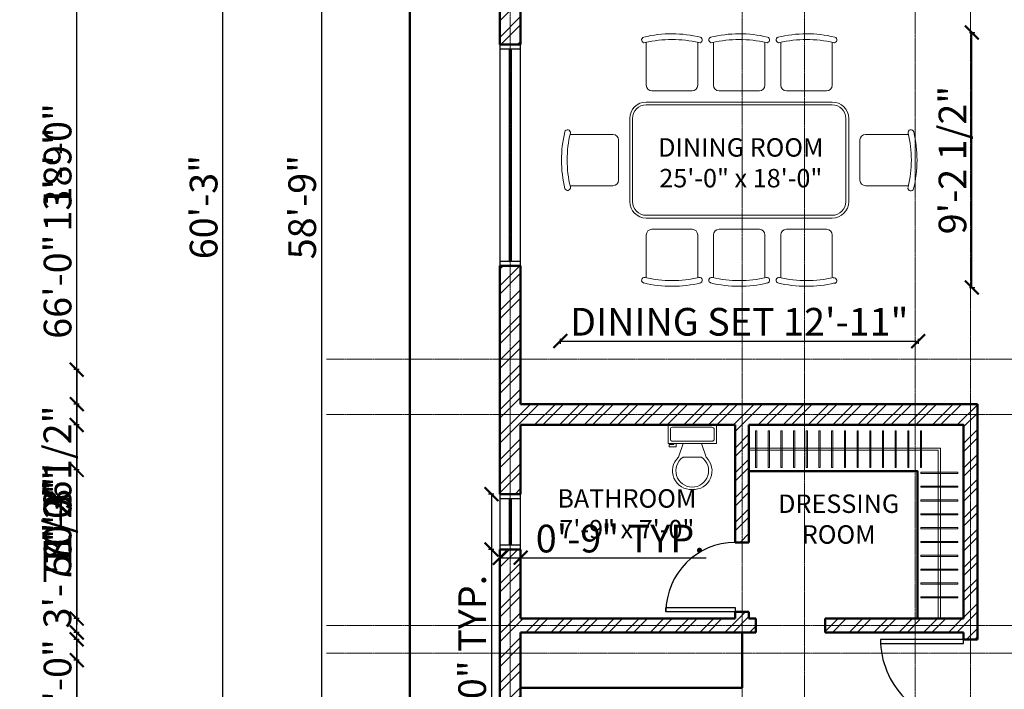
# Model space of a CAD drawing. Units: inches. Extents: x 261 to 2725, y 291 to 1454.
# Tile 6 of 35: x 261 to 688, y 661 to 951. Entities that reach past the tile are written whole.
import ezdxf

# ---------------------------------------------------------------- set-up
doc = ezdxf.new("R2010")
doc.units = ezdxf.units.IN
doc.linetypes.add('CENTER', pattern=[2, 1.25, -0.25, 0.25, -0.25])
for name, color, linetype, lineweight in [('A-ANNO-DIMS', 136, 'Continuous', 18), ('A-AREA-IDEN', 18, 'Continuous', 18), ('A-DOOR', 160, 'Continuous', 25), ('A-FLOR-FIXT', 145, 'Continuous', 18), ('A-FURN', 30, 'Continuous', 18), ('A-GLAZ', 150, 'Continuous', 25), ('A-GRID', 251, 'CENTER', 13), ('A-WALL', 222, 'Continuous', 50), ('A-WALL-PATT', 243, 'Continuous', 13)]:
    doc.layers.add(name, color=color, linetype=linetype, lineweight=lineweight)
doc.styles.get("Standard").update_dxf_attribs({"font": 'arial.ttf'})
doc.dimstyles.new('ISO-25', dxfattribs={"dimtxt": 12, "dimasz": 6, "dimexe": 1.25, "dimexo": 0.625, "dimtad": 1, "dimdec": 0, "dimlunit": 3, "dimtxsty": 'Standard', "dimblk": 'ARCHTICK', "dimcen": 2.5, "dimadec": 0, "dimazin": 0, "dimtfac": 1, "dimtdec": 0, "dimtmove": 0, "dimatfit": 3, "dimfxl": 1, "dimfxlon": 1, "dimarcsym": 0})

# ---------------------------------------------------------------- blocks, each defined once
blk = doc.blocks.new('*U5')
for p, q in [((0, 0), (0, -4)), ((-36, 0), (-36, -4))]:
    blk.add_line(p, q)
blk.add_lwpolyline([(0, 0), (0, 36), (-1.75, 36), (-1.75, 0)], close=True)
blk.add_arc((0, 0), 36, 90, 180)
blk = doc.blocks.new('*U3')
for p, q in [((0, 0), (0, -6)), ((30, 0), (30, -6))]:
    blk.add_line(p, q)
blk.add_lwpolyline([(0, 0), (0, 30), (1.75, 30), (1.75, 0)], close=True)
blk.add_arc((0, 0), 30, 0, 90)
blk = doc.blocks.new('A$C593F2FDE')
for p, q in [((0.8501, 2.0223), (0.8501, 2.4542)), ((1.3676, 2.0223), (1.3676, 2.4542)), ((1.5273, 2.0223), (1.5273, 2.4542)), ((2.0448, 2.0223), (2.0448, 2.4542)), ((2.2045, 2.0223), (2.2045, 2.4542)), ((2.722, 2.0223), (2.722, 2.4542)), ((0.9063, 1.966), (1.3113, 1.966)), ((1.9885, 1.966), (1.5835, 1.966)), ((2.6658, 1.966), (2.2608, 1.966)), ((0.85, 1.8535), (2.722, 1.8535)), ((0.85, 1.825), (2.722, 1.825)), ((0.6835, 1.687), (0.6835, 0.85)), ((0.7121, 1.687), (0.7121, 0.85)), ((2.86, 1.687), (2.86, 0.85)), ((2.8885, 1.687), (2.8885, 0.85)), ((0.5148, 1.5273), (0.0828, 1.5273)), ((3.0573, 1.5273), (3.4892, 1.5273)), ((0.571, 1.471), (0.571, 1.066)), ((3.001, 1.471), (3.001, 1.066)), ((0.5148, 1.0098), (0.0828, 1.0098)), ((3.0573, 1.0098), (3.4892, 1.0098)), ((0.85, 0.7121), (2.722, 0.7121)), ((0.85, 0.6835), (2.722, 0.6835)), ((0.8501, 0.5148), (0.8501, 0.0828)), ((0.9063, 0.571), (1.3113, 0.571)), ((1.3676, 0.5148), (1.3676, 0.0828)), ((1.5273, 0.5148), (1.5273, 0.0828)), ((1.9885, 0.571), (1.5835, 0.571)), ((2.0448, 0.5148), (2.0448, 0.0828)), ((2.2045, 0.5148), (2.2045, 0.0828)), ((2.6658, 0.571), (2.2608, 0.571)), ((2.722, 0.5148), (2.722, 0.0828))]:
    blk.add_line(p, q)
for centre, radius, start, end in [((0.8316, 2.4793), 0.0286, 102.88207, 282.88207), ((1.1088, 1.3263), 1.2144, 76.2483, 103.50545), ((1.1088, 1.3263), 1.1572, 76.46376, 103.53624), ((1.386, 2.4793), 0.0286, 257.11793, 77.11793), ((1.5088, 2.4793), 0.0286, 102.88207, 282.88207), ((1.786, 1.3263), 1.2144, 76.49455, 103.7517), ((1.786, 1.3263), 1.1572, 76.46376, 103.53624), ((2.0633, 2.4793), 0.0286, 257.11793, 77.11793), ((2.186, 2.4793), 0.0286, 102.88207, 282.88207), ((2.4633, 1.3263), 1.2144, 76.49455, 103.7517), ((2.4633, 1.3263), 1.1572, 76.46376, 103.53624), ((2.7405, 2.4793), 0.0286, 257.11793, 77.11793), ((0.9063, 2.0223), 0.0563, 180, 270), ((1.3113, 2.0223), 0.0563, 270, 0), ((1.5835, 2.0223), 0.0563, 180, 270), ((1.9885, 2.0223), 0.0563, 270, 0), ((2.2608, 2.0223), 0.0563, 180, 270), ((2.6658, 2.0223), 0.0563, 270, 0), ((0.85, 1.687), 0.1665, 90, 180), ((0.85, 1.687), 0.1379, 90, 180), ((2.722, 1.687), 0.1665, 0, 90), ((2.722, 1.687), 0.1379, 0, 90), ((1.2108, 1.2685), 1.2144, 166.49455, 193.7517), ((0.0578, 1.5458), 0.0286, 347.11793, 167.11793), ((1.2108, 1.2685), 1.1572, 166.46376, 193.53624), ((0.5148, 1.471), 0.0563, 0, 90), ((3.0573, 1.471), 0.0563, 90, 180), ((3.5143, 1.5458), 0.0286, 12.88207, 192.88207), ((2.3613, 1.2685), 1.1572, 346.46376, 13.53624), ((2.3613, 1.2685), 1.2144, 346.2483, 13.50545), ((0.0578, 0.9913), 0.0286, 192.88207, 12.88207), ((0.5148, 1.066), 0.0563, 270, 0), ((3.0573, 1.066), 0.0563, 180, 270), ((3.513, 0.9862), 0.0286, 167.11793, 347.11793), ((0.85, 0.85), 0.1665, 180, 270), ((0.85, 0.85), 0.1379, 180, 270), ((2.722, 0.85), 0.1665, 270, 0), ((2.722, 0.85), 0.1379, 270, 0), ((0.9063, 0.5148), 0.0563, 90, 180), ((1.3113, 0.5148), 0.0563, 0, 90), ((1.5835, 0.5148), 0.0563, 90, 180), ((1.9885, 0.5148), 0.0563, 0, 90), ((2.2608, 0.5148), 0.0563, 90, 180), ((2.6658, 0.5148), 0.0563, 0, 90), ((0.8316, 0.0578), 0.0286, 77.11793, 257.11793), ((1.1088, 1.2108), 1.2144, 256.49455, 283.7517), ((1.1088, 1.2108), 1.1572, 256.46376, 283.53624), ((1.386, 0.0578), 0.0286, 282.88207, 102.88207), ((1.5088, 0.0578), 0.0286, 77.11793, 257.11793), ((1.786, 1.2108), 1.2144, 256.2483, 283.50545), ((1.786, 1.2108), 1.1572, 256.46376, 283.53624), ((2.0633, 0.0578), 0.0286, 282.88207, 102.88207), ((2.186, 0.0578), 0.0286, 77.11793, 257.11793), ((2.4633, 1.2108), 1.2144, 256.2483, 283.50545), ((2.4633, 1.2108), 1.1572, 256.46376, 283.53624), ((2.7393, 0.0528), 0.0286, 282.88207, 102.88207)]:
    blk.add_arc(centre, radius, start, end)
blk = doc.blocks.new('*U27')
for p, q in [((9.5, -6), (9.5, -2)), ((-10, -8.5), (-8, -8.5)), ((-10, -9.5), (-10, -8.5)), ((-8, -8.5), (-8, -8)), ((-7, -8), (-7, -9.5)), ((-4, -8), (-6, -14)), ((4, -8), (6, -14)), ((-7, -9.5), (-10, -9.5)), ((4, -14), (-4, -14))]:
    blk.add_line(p, q)
blk.add_lwpolyline([(10.5, -8), (10.5, 0), (-10.5, 0), (-10.5, -8)], close=True)
for points in [[(-9.5, -2), (-9.5, -6)], [(8.5, -1), (-8.5, -1)], [(-8.5, -7), (8.5, -7)]]:
    blk.add_lwpolyline(points)
for centre, radius, start, end in [((-8.625, -1.875), 0.8839, 81.8699, 188.1301), ((8.625, -1.875), 0.8839, 351.8699, 98.1301), ((-8.625, -6.125), 0.8839, 171.869898, 278.1301), ((8.625, -6.125), 0.8839, 261.8699, 8.1301), ((-0.4772, -19.9188), 8.0953, 133.01722, 273.38), ((0.0374, -19.8731), 7.127, 124.50543, 269.7), ((-0.0373, -19.8731), 7.127, 270.3, 55.4946), ((0.4773, -19.9188), 8.0953, 266.62, 46.9828)]:
    blk.add_arc(centre, radius, start, end)
blk = doc.blocks.new('_ArchTick')
at = {"color": 0, "linetype": 'ByBlock', "const_width": 0.15}
blk.add_lwpolyline([(-0.5, -0.5), (0.5, 0.5)], dxfattribs=at)
blk = doc.blocks.new('*D29')
at = {"layer": 'A-ANNO-DIMS', "color": 0, "lineweight": -2, "transparency": 16777216}
for p, q in [((350.37, 1231.47), (348.12, 1231.47)), ((349.37, 508.47), (349.37, 1231.47)), ((350.37, 508.47), (348.12, 508.47))]:
    blk.add_line(p, q, dxfattribs=at)
at = {"layer": 'Defpoints', "color": 0, "transparency": 16777216}
for p in [(349.37, 1231.47), (469.45, 1231.47), (469.45, 508.47)]:
    blk.add_point(p, dxfattribs=at)
at = {"layer": 'A-ANNO-DIMS', "color": 0, "lineweight": -2, "transparency": 16777216, "xscale": 6, "yscale": 6, "zscale": 6}
for p, rotation in [((349.37, 1231.47), 90), ((349.37, 508.47), 270)]:
    blk.add_blockref('_ArchTick', p, dxfattribs=dict(at, rotation=rotation))
at = {"layer": 'A-ANNO-DIMS', "color": 0, "transparency": 16777216, "insert": (342.61, 869.97), "char_height": 12, "attachment_point": 5, "rotation": 90}
blk.add_mtext('60\'-3"', dxfattribs=at)
blk = doc.blocks.new('*D30')
at = {"layer": 'A-ANNO-DIMS', "color": 0, "lineweight": -2, "transparency": 16777216}
for p, q in [((393.09, 1222.47), (390.84, 1222.47)), ((392.09, 1222.47), (392.09, 517.47)), ((393.09, 517.47), (390.84, 517.47))]:
    blk.add_line(p, q, dxfattribs=at)
at = {"layer": 'Defpoints', "color": 0, "transparency": 16777216}
for p in [(478.45, 1222.47), (392.09, 517.47), (478.45, 517.47)]:
    blk.add_point(p, dxfattribs=at)
at = {"layer": 'A-ANNO-DIMS', "color": 0, "lineweight": -2, "transparency": 16777216, "xscale": 6, "yscale": 6, "zscale": 6}
for p, rotation in [((392.09, 1222.47), 90), ((392.09, 517.47), 270)]:
    blk.add_blockref('_ArchTick', p, dxfattribs=dict(at, rotation=rotation))
at = {"layer": 'A-ANNO-DIMS', "color": 0, "transparency": 16777216, "insert": (385.34, 869.97), "char_height": 12, "attachment_point": 5, "rotation": 90}
blk.add_mtext('58\'-9"', dxfattribs=at)
blk = doc.blocks.new('WIN-24')
for p, q in [((1455.08, 973.47), (1455.08, 964.47)), ((1475.08, 964.47), (1475.08, 973.47)), ((1475.08, 969.47), (1455.08, 969.47)), ((1455.08, 968.47), (1475.08, 968.47))]:
    blk.add_line(p, q)
blk.add_lwpolyline([(1477.08, 964.47), (1477.08, 973.47), (1453.08, 973.47), (1453.08, 964.47)], close=True)
blk = doc.blocks.new('*D61')
at = {"layer": 'A-ANNO-DIMS', "color": 0, "lineweight": -2, "ltscale": 0.07, "transparency": 16777216}
for p, q in [((466.85, 745.47), (464.6, 745.47)), ((465.85, 745.47), (465.85, 721.47)), ((466.85, 721.47), (464.6, 721.47)), ((465.85, 721.47), (465.85, 532.56))]:
    blk.add_line(p, q, dxfattribs=at)
at = {"layer": 'Defpoints', "color": 0, "ltscale": 0.07, "transparency": 16777216}
for p in [(469.45, 745.47), (465.85, 721.47), (469.45, 721.47)]:
    blk.add_point(p, dxfattribs=at)
at = {"layer": 'A-ANNO-DIMS', "color": 0, "lineweight": -2, "ltscale": 0.07, "transparency": 16777216, "xscale": 6, "yscale": 6, "zscale": 6}
for p, rotation in [((465.85, 745.47), 90), ((465.85, 721.47), 270)]:
    blk.add_blockref('_ArchTick', p, dxfattribs=dict(at, rotation=rotation))
at = {"layer": 'A-ANNO-DIMS', "color": 0, "ltscale": 0.07, "transparency": 16777216, "insert": (459.02, 624.02), "char_height": 12, "attachment_point": 5, "rotation": 90}
blk.add_mtext('WINDOW W4 2\'-0" TYP.', dxfattribs=at)
blk = doc.blocks.new('*D62')
at = {"layer": 'A-ANNO-DIMS', "color": 0, "lineweight": -2, "ltscale": 0.07, "transparency": 16777216}
for p, q in [((469.45, 718.87), (469.45, 716.62)), ((469.45, 717.87), (478.45, 717.87)), ((478.45, 718.87), (478.45, 716.62)), ((478.45, 717.87), (558.85, 717.87))]:
    blk.add_line(p, q, dxfattribs=at)
at = {"layer": 'Defpoints', "color": 0, "ltscale": 0.07, "transparency": 16777216}
for p in [(469.45, 721.47), (478.45, 721.47), (478.45, 717.87)]:
    blk.add_point(p, dxfattribs=at)
at = {"layer": 'A-ANNO-DIMS', "color": 0, "lineweight": -2, "ltscale": 0.07, "transparency": 16777216, "xscale": 6, "yscale": 6, "zscale": 6, "rotation": 180}
blk.add_blockref('_ArchTick', (469.45, 717.87), dxfattribs=at)
at = {"layer": 'A-ANNO-DIMS', "color": 0, "lineweight": -2, "ltscale": 0.07, "transparency": 16777216, "xscale": 6, "yscale": 6, "zscale": 6}
blk.add_blockref('_ArchTick', (478.45, 717.87), dxfattribs=at)
at = {"layer": 'A-ANNO-DIMS', "color": 0, "ltscale": 0.07, "transparency": 16777216, "insert": (521.65, 724.62), "char_height": 12, "attachment_point": 5}
blk.add_mtext('0\'-9" TYP.', dxfattribs=at)
blk = doc.blocks.new('*D65')
at = {"layer": 'A-ANNO-DIMS', "color": 0, "lineweight": -2, "ltscale": 0.07, "transparency": 16777216}
for p, q in [((495.67, 812.84), (495.67, 810.59)), ((495.67, 811.84), (650.78, 811.84)), ((650.78, 812.84), (650.78, 810.59))]:
    blk.add_line(p, q, dxfattribs=at)
at = {"layer": 'Defpoints', "color": 0, "ltscale": 0.07, "transparency": 16777216}
for p in [(495.67, 835.11), (650.78, 835.11), (650.78, 811.84)]:
    blk.add_point(p, dxfattribs=at)
at = {"layer": 'A-ANNO-DIMS', "color": 0, "lineweight": -2, "ltscale": 0.07, "transparency": 16777216, "xscale": 6, "yscale": 6, "zscale": 6, "rotation": 180}
blk.add_blockref('_ArchTick', (495.67, 811.84), dxfattribs=at)
at = {"layer": 'A-ANNO-DIMS', "color": 0, "lineweight": -2, "ltscale": 0.07, "transparency": 16777216, "xscale": 6, "yscale": 6, "zscale": 6}
blk.add_blockref('_ArchTick', (650.78, 811.84), dxfattribs=at)
at = {"layer": 'A-ANNO-DIMS', "color": 0, "ltscale": 0.07, "transparency": 16777216, "insert": (573.23, 818.67), "char_height": 12, "attachment_point": 5}
blk.add_mtext('DINING SET 12\'-11"', dxfattribs=at)
blk = doc.blocks.new('*D66')
at = {"layer": 'A-ANNO-DIMS', "color": 0, "lineweight": -2, "ltscale": 0.07, "transparency": 16777216}
for p, q in [((673.05, 945.66), (675.3, 945.66)), ((674.05, 835.11), (674.05, 945.66)), ((673.05, 835.11), (675.3, 835.11))]:
    blk.add_line(p, q, dxfattribs=at)
at = {"layer": 'Defpoints', "color": 0, "ltscale": 0.07, "transparency": 16777216}
for p in [(650.78, 945.66), (674.05, 945.66), (650.78, 835.11)]:
    blk.add_point(p, dxfattribs=at)
at = {"layer": 'A-ANNO-DIMS', "color": 0, "lineweight": -2, "ltscale": 0.07, "transparency": 16777216, "xscale": 6, "yscale": 6, "zscale": 6}
for p, rotation in [((674.05, 945.66), 90), ((674.05, 835.11), 270)]:
    blk.add_blockref('_ArchTick', p, dxfattribs=dict(at, rotation=rotation))
at = {"layer": 'A-ANNO-DIMS', "color": 0, "ltscale": 0.07, "transparency": 16777216, "insert": (667.22, 890.38), "char_height": 12, "attachment_point": 5, "rotation": 90}
blk.add_mtext('9\'-2 1/2"', dxfattribs=at)
blk = doc.blocks.new('*D77')
at = {"layer": 'A-ANNO-DIMS', "color": 0, "lineweight": -2, "ltscale": 0.07, "transparency": 16777216}
for p, q in [((287.06, 685.47), (284.81, 685.47)), ((286.06, 517.47), (286.06, 685.47)), ((287.06, 517.47), (284.81, 517.47))]:
    blk.add_line(p, q, dxfattribs=at)
at = {"layer": 'Defpoints', "color": 0, "ltscale": 0.07, "transparency": 16777216}
for p in [(286.06, 685.47), (478.45, 685.47), (478.45, 517.47)]:
    blk.add_point(p, dxfattribs=at)
at = {"layer": 'A-ANNO-DIMS', "color": 0, "lineweight": -2, "ltscale": 0.07, "transparency": 16777216, "xscale": 6, "yscale": 6, "zscale": 6}
for p, rotation in [((286.06, 685.47), 90), ((286.06, 517.47), 270)]:
    blk.add_blockref('_ArchTick', p, dxfattribs=dict(at, rotation=rotation))
at = {"layer": 'A-ANNO-DIMS', "color": 0, "ltscale": 0.07, "transparency": 16777216, "insert": (279.3, 601.47), "char_height": 12, "attachment_point": 5, "rotation": 90}
blk.add_mtext('14\'-0"', dxfattribs=at)
blk = doc.blocks.new('*D78')
at = {"layer": 'A-ANNO-DIMS', "color": 0, "lineweight": -2, "ltscale": 0.07, "transparency": 16777216}
for p, q in [((287.06, 784.47), (284.81, 784.47)), ((286.06, 685.47), (286.06, 784.47)), ((287.06, 685.47), (284.81, 685.47))]:
    blk.add_line(p, q, dxfattribs=at)
at = {"layer": 'Defpoints', "color": 0, "ltscale": 0.07, "transparency": 16777216}
for p in [(286.06, 784.47), (478.45, 784.47), (478.45, 685.47)]:
    blk.add_point(p, dxfattribs=at)
at = {"layer": 'A-ANNO-DIMS', "color": 0, "lineweight": -2, "ltscale": 0.07, "transparency": 16777216, "xscale": 6, "yscale": 6, "zscale": 6}
for p, rotation in [((286.06, 784.47), 90), ((286.06, 685.47), 270)]:
    blk.add_blockref('_ArchTick', p, dxfattribs=dict(at, rotation=rotation))
at = {"layer": 'A-ANNO-DIMS', "color": 0, "ltscale": 0.07, "transparency": 16777216, "insert": (279.3, 734.97), "char_height": 12, "attachment_point": 5, "rotation": 90}
blk.add_mtext('8\'-3"', dxfattribs=at)
blk = doc.blocks.new('*D79')
at = {"layer": 'A-ANNO-DIMS', "color": 0, "lineweight": -2, "ltscale": 0.07, "transparency": 16777216}
for p, q in [((287.06, 1000.47), (284.81, 1000.47)), ((286.06, 784.47), (286.06, 1000.47)), ((287.06, 784.47), (284.81, 784.47))]:
    blk.add_line(p, q, dxfattribs=at)
at = {"layer": 'Defpoints', "color": 0, "ltscale": 0.07, "transparency": 16777216}
for p in [(286.06, 1000.47), (478.45, 1000.47), (478.45, 784.47)]:
    blk.add_point(p, dxfattribs=at)
at = {"layer": 'A-ANNO-DIMS', "color": 0, "lineweight": -2, "ltscale": 0.07, "transparency": 16777216, "xscale": 6, "yscale": 6, "zscale": 6}
for p, rotation in [((286.06, 1000.47), 90), ((286.06, 784.47), 270)]:
    blk.add_blockref('_ArchTick', p, dxfattribs=dict(at, rotation=rotation))
at = {"layer": 'A-ANNO-DIMS', "color": 0, "ltscale": 0.07, "transparency": 16777216, "insert": (279.3, 892.47), "char_height": 12, "attachment_point": 5, "rotation": 90}
blk.add_mtext('18\'-0"', dxfattribs=at)
blk = doc.blocks.new('*D86')
at = {"layer": 'A-ANNO-DIMS', "color": 0, "lineweight": -2, "ltscale": 0.07, "transparency": 16777216}
for p, q in [((676.45, 1437.76), (676.45, 1440.01)), ((676.45, 1438.76), (772.45, 1438.76)), ((772.45, 1437.76), (772.45, 1440.01))]:
    blk.add_line(p, q, dxfattribs=at)
at = {"layer": 'Defpoints', "color": 0, "ltscale": 0.07, "transparency": 16777216}
for p in [(772.45, 1438.76), (676.45, 517.47), (772.45, 517.47)]:
    blk.add_point(p, dxfattribs=at)
at = {"layer": 'A-ANNO-DIMS', "color": 0, "lineweight": -2, "ltscale": 0.07, "transparency": 16777216, "xscale": 6, "yscale": 6, "zscale": 6, "rotation": 180}
blk.add_blockref('_ArchTick', (676.45, 1438.76), dxfattribs=at)
at = {"layer": 'A-ANNO-DIMS', "color": 0, "lineweight": -2, "ltscale": 0.07, "transparency": 16777216, "xscale": 6, "yscale": 6, "zscale": 6}
blk.add_blockref('_ArchTick', (772.45, 1438.76), dxfattribs=at)
at = {"layer": 'A-ANNO-DIMS', "color": 0, "ltscale": 0.07, "transparency": 16777216, "insert": (724.45, 1445.51), "char_height": 12, "attachment_point": 5}
blk.add_mtext('8\'-0"', dxfattribs=at)
blk = doc.blocks.new('*D96')
at = {"layer": 'A-ANNO-DIMS', "color": 0, "lineweight": -2, "ltscale": 0.07, "transparency": 16777216}
for p, q in [((577.45, 305.22), (577.45, 302.97)), ((577.45, 304.22), (670.45, 304.22)), ((670.45, 305.22), (670.45, 302.97))]:
    blk.add_line(p, q, dxfattribs=at)
at = {"layer": 'Defpoints', "color": 0, "ltscale": 0.07, "transparency": 16777216}
for p in [(577.45, 775.47), (670.45, 775.47), (670.45, 304.22)]:
    blk.add_point(p, dxfattribs=at)
at = {"layer": 'A-ANNO-DIMS', "color": 0, "lineweight": -2, "ltscale": 0.07, "transparency": 16777216, "xscale": 6, "yscale": 6, "zscale": 6, "rotation": 180}
blk.add_blockref('_ArchTick', (577.45, 304.22), dxfattribs=at)
at = {"layer": 'A-ANNO-DIMS', "color": 0, "lineweight": -2, "ltscale": 0.07, "transparency": 16777216, "xscale": 6, "yscale": 6, "zscale": 6}
blk.add_blockref('_ArchTick', (670.45, 304.22), dxfattribs=at)
at = {"layer": 'A-ANNO-DIMS', "color": 0, "ltscale": 0.07, "transparency": 16777216, "insert": (623.95, 310.97), "char_height": 12, "attachment_point": 5}
blk.add_mtext('7\'-9"', dxfattribs=at)
blk = doc.blocks.new('*D97')
at = {"layer": 'A-ANNO-DIMS', "color": 0, "lineweight": -2, "ltscale": 0.07, "transparency": 16777216}
for p, q in [((287.06, 775.47), (284.81, 775.47)), ((286.06, 775.47), (286.06, 691.47)), ((287.06, 691.47), (284.81, 691.47))]:
    blk.add_line(p, q, dxfattribs=at)
at = {"layer": 'Defpoints', "color": 0, "ltscale": 0.07, "transparency": 16777216}
for p in [(670.45, 775.47), (286.06, 691.47), (670.45, 691.47)]:
    blk.add_point(p, dxfattribs=at)
at = {"layer": 'A-ANNO-DIMS', "color": 0, "lineweight": -2, "ltscale": 0.07, "transparency": 16777216, "xscale": 6, "yscale": 6, "zscale": 6}
for p, rotation in [((286.06, 775.47), 90), ((286.06, 691.47), 270)]:
    blk.add_blockref('_ArchTick', p, dxfattribs=dict(at, rotation=rotation))
at = {"layer": 'A-ANNO-DIMS', "color": 0, "ltscale": 0.07, "transparency": 16777216, "insert": (279.3, 733.47), "char_height": 12, "attachment_point": 5, "rotation": 90}
blk.add_mtext('7\'-0"', dxfattribs=at)
blk = doc.blocks.new('*D98')
at = {"layer": 'A-ANNO-DIMS', "color": 0, "lineweight": -2, "ltscale": 0.07, "transparency": 16777216}
for p, q in [((287.06, 682.47), (284.81, 682.47)), ((286.06, 682.47), (286.06, 646.47)), ((287.06, 646.47), (284.81, 646.47))]:
    blk.add_line(p, q, dxfattribs=at)
at = {"layer": 'Defpoints', "color": 0, "ltscale": 0.07, "transparency": 16777216}
for p in [(676.45, 682.47), (286.06, 646.47), (676.45, 646.47)]:
    blk.add_point(p, dxfattribs=at)
at = {"layer": 'A-ANNO-DIMS', "color": 0, "lineweight": -2, "ltscale": 0.07, "transparency": 16777216, "xscale": 6, "yscale": 6, "zscale": 6}
for p, rotation in [((286.06, 682.47), 90), ((286.06, 646.47), 270)]:
    blk.add_blockref('_ArchTick', p, dxfattribs=dict(at, rotation=rotation))
at = {"layer": 'A-ANNO-DIMS', "color": 0, "ltscale": 0.07, "transparency": 16777216, "insert": (279.3, 664.47), "char_height": 12, "attachment_point": 5, "rotation": 90}
blk.add_mtext('3\'-0"', dxfattribs=at)
blk = doc.blocks.new('*D100')
at = {"layer": 'A-ANNO-DIMS', "color": 0, "lineweight": -2, "ltscale": 0.07, "transparency": 16777216}
for p, q in [((287.06, 799.47), (284.81, 799.47)), ((286.06, 799.47), (286.06, 755.97)), ((287.06, 755.97), (284.81, 755.97)), ((286.06, 755.97), (286.06, 688.87))]:
    blk.add_line(p, q, dxfattribs=at)
at = {"layer": 'Defpoints', "color": 0, "ltscale": 0.07, "transparency": 16777216}
for p in [(825.95, 799.47), (286.06, 755.97), (825.95, 755.97)]:
    blk.add_point(p, dxfattribs=at)
at = {"layer": 'A-ANNO-DIMS', "color": 0, "lineweight": -2, "ltscale": 0.07, "transparency": 16777216, "xscale": 6, "yscale": 6, "zscale": 6}
for p, rotation in [((286.06, 799.47), 90), ((286.06, 755.97), 270)]:
    blk.add_blockref('_ArchTick', p, dxfattribs=dict(at, rotation=rotation))
at = {"layer": 'A-ANNO-DIMS', "color": 0, "ltscale": 0.07, "transparency": 16777216, "insert": (279.22, 719.42), "char_height": 12, "attachment_point": 5, "rotation": 90}
blk.add_mtext('3\'-7 1/2"', dxfattribs=at)
blk = doc.blocks.new('*D103')
at = {"layer": 'A-ANNO-DIMS', "color": 0, "lineweight": -2, "ltscale": 0.07, "transparency": 16777216}
for p, q in [((287.06, 1231.47), (284.81, 1231.47)), ((286.06, 439.47), (286.06, 1231.47)), ((287.06, 439.47), (284.81, 439.47))]:
    blk.add_line(p, q, dxfattribs=at)
at = {"layer": 'Defpoints', "color": 0, "ltscale": 0.07, "transparency": 16777216}
for p in [(286.06, 1231.47), (1243.08, 1231.47), (1243.08, 439.47)]:
    blk.add_point(p, dxfattribs=at)
at = {"layer": 'A-ANNO-DIMS', "color": 0, "lineweight": -2, "ltscale": 0.07, "transparency": 16777216, "xscale": 6, "yscale": 6, "zscale": 6}
for p, rotation in [((286.06, 1231.47), 90), ((286.06, 439.47), 270)]:
    blk.add_blockref('_ArchTick', p, dxfattribs=dict(at, rotation=rotation))
at = {"layer": 'A-ANNO-DIMS', "color": 0, "ltscale": 0.07, "transparency": 16777216, "insert": (279.3, 835.47), "char_height": 12, "attachment_point": 5, "rotation": 90}
blk.add_mtext('66\'-0"', dxfattribs=at)
blk = doc.blocks.new('*D107')
at = {"layer": 'A-ANNO-DIMS', "color": 0, "lineweight": -2, "ltscale": 0.07, "transparency": 16777216}
for p, q in [((287.06, 673.47), (284.81, 673.47)), ((286.06, 496.47), (286.06, 673.47)), ((287.06, 496.47), (284.81, 496.47))]:
    blk.add_line(p, q, dxfattribs=at)
at = {"layer": 'Defpoints', "color": 0, "ltscale": 0.07, "transparency": 16777216}
for p in [(286.06, 673.47), (1252.08, 673.47), (1252.08, 496.47)]:
    blk.add_point(p, dxfattribs=at)
at = {"layer": 'A-ANNO-DIMS', "color": 0, "lineweight": -2, "ltscale": 0.07, "transparency": 16777216, "xscale": 6, "yscale": 6, "zscale": 6}
for p, rotation in [((286.06, 673.47), 90), ((286.06, 496.47), 270)]:
    blk.add_blockref('_ArchTick', p, dxfattribs=dict(at, rotation=rotation))
at = {"layer": 'A-ANNO-DIMS', "color": 0, "ltscale": 0.07, "transparency": 16777216, "insert": (279.3, 584.97), "char_height": 12, "attachment_point": 5, "rotation": 90}
blk.add_mtext('14\'-9"', dxfattribs=at)
blk = doc.blocks.new('*D108')
at = {"layer": 'A-ANNO-DIMS', "color": 0, "lineweight": -2, "ltscale": 0.07, "transparency": 16777216}
for p, q in [((287.06, 799.47), (284.81, 799.47)), ((286.06, 673.47), (286.06, 799.47)), ((287.06, 673.47), (284.81, 673.47))]:
    blk.add_line(p, q, dxfattribs=at)
at = {"layer": 'Defpoints', "color": 0, "ltscale": 0.07, "transparency": 16777216}
for p in [(286.06, 799.47), (1252.08, 799.47), (1252.08, 673.47)]:
    blk.add_point(p, dxfattribs=at)
at = {"layer": 'A-ANNO-DIMS', "color": 0, "lineweight": -2, "ltscale": 0.07, "transparency": 16777216, "xscale": 6, "yscale": 6, "zscale": 6}
for p, rotation in [((286.06, 799.47), 90), ((286.06, 673.47), 270)]:
    blk.add_blockref('_ArchTick', p, dxfattribs=dict(at, rotation=rotation))
at = {"layer": 'A-ANNO-DIMS', "color": 0, "ltscale": 0.07, "transparency": 16777216, "insert": (279.3, 736.47), "char_height": 12, "attachment_point": 5, "rotation": 90}
blk.add_mtext('10\'-6"', dxfattribs=at)
blk = doc.blocks.new('*D109')
at = {"layer": 'A-ANNO-DIMS', "color": 0, "lineweight": -2, "ltscale": 0.07, "transparency": 16777216}
for p, q in [((287.06, 964.47), (284.81, 964.47)), ((286.06, 799.47), (286.06, 964.47)), ((287.06, 799.47), (284.81, 799.47))]:
    blk.add_line(p, q, dxfattribs=at)
at = {"layer": 'Defpoints', "color": 0, "ltscale": 0.07, "transparency": 16777216}
for p in [(286.06, 964.47), (1252.08, 964.47), (1252.08, 799.47)]:
    blk.add_point(p, dxfattribs=at)
at = {"layer": 'A-ANNO-DIMS', "color": 0, "lineweight": -2, "ltscale": 0.07, "transparency": 16777216, "xscale": 6, "yscale": 6, "zscale": 6}
for p, rotation in [((286.06, 964.47), 90), ((286.06, 799.47), 270)]:
    blk.add_blockref('_ArchTick', p, dxfattribs=dict(at, rotation=rotation))
at = {"layer": 'A-ANNO-DIMS', "color": 0, "ltscale": 0.07, "transparency": 16777216, "insert": (279.3, 881.97), "char_height": 12, "attachment_point": 5, "rotation": 90}
blk.add_mtext('13\'-9"', dxfattribs=at)
blk = doc.blocks.new('*D123')
at = {"layer": 'A-ANNO-DIMS', "color": 0, "lineweight": -2, "ltscale": 0.07, "transparency": 16777216}
for p, q in [((287.06, 1054.85), (284.81, 1054.85)), ((286.06, 439.47), (286.06, 1054.85)), ((287.06, 439.47), (284.81, 439.47))]:
    blk.add_line(p, q, dxfattribs=at)
at = {"layer": 'Defpoints', "color": 0, "ltscale": 0.07, "transparency": 16777216}
for p in [(286.06, 1054.85), (2007.71, 1054.85), (2007.71, 439.47)]:
    blk.add_point(p, dxfattribs=at)
at = {"layer": 'A-ANNO-DIMS', "color": 0, "lineweight": -2, "ltscale": 0.07, "transparency": 16777216, "xscale": 6, "yscale": 6, "zscale": 6}
for p, rotation in [((286.06, 1054.85), 90), ((286.06, 439.47), 270)]:
    blk.add_blockref('_ArchTick', p, dxfattribs=dict(at, rotation=rotation))
at = {"layer": 'A-ANNO-DIMS', "color": 0, "ltscale": 0.07, "transparency": 16777216, "insert": (279.22, 747.16), "char_height": 12, "attachment_point": 5, "rotation": 90}
blk.add_mtext('51\'-3 1/2"', dxfattribs=at)

msp = doc.modelspace()

# ---------------------------------------------------------------- hatches: boundary and pattern name
at = {"layer": 'A-WALL-PATT'}
h = msp.add_hatch(dxfattribs=at)
h.set_pattern_fill('ANSI32', color=256, scale=0.8)
h.paths.add_polyline_path([(478.45, 685.47), (580.45, 685.47), (580.45, 691.47), (577.45, 691.47), (577.45, 694.47), (571.45, 694.47), (571.45, 691.47), (478.45, 691.47), (478.45, 721.47), (469.45, 721.47), (469.45, 508.47), (538.45, 508.47), (538.45, 517.47), (478.45, 517.47)])
h.paths.add_polyline_path([(694.45, 517.47), (676.45, 517.47), (676.45, 646.47), (670.45, 646.47), (670.45, 517.47), (610.45, 517.47), (610.45, 508.47), (694.45, 508.47)])
h.paths.add_polyline_path([(676.45, 784.47), (478.45, 784.47), (478.45, 844.47), (469.45, 844.47), (469.45, 745.47), (478.45, 745.47), (478.45, 775.47), (571.45, 775.47), (571.45, 724.47), (577.45, 724.47), (577.45, 775.47), (670.45, 775.47), (670.45, 691.47), (610.45, 691.47), (610.45, 685.47), (670.45, 685.47), (670.45, 682.47), (676.45, 682.47)])
h.paths.add_polyline_path([(955.45, 880.47), (946.45, 880.47), (946.45, 808.47), (778.45, 808.47), (778.45, 799.47), (946.45, 799.47), (946.45, 517.47), (898.45, 517.47), (898.45, 508.47), (955.45, 508.47)])
h.paths.add_polyline_path([(778.45, 598.47), (772.45, 598.47), (772.45, 517.47), (754.45, 517.47), (754.45, 508.47), (826.45, 508.47), (826.45, 517.47), (778.45, 517.47)])
h.paths.add_polyline_path([(955.45, 1090.47), (946.45, 1090.47), (946.45, 1030.47), (817.45, 1030.47), (817.45, 1024.47), (946.45, 1024.47), (946.45, 952.47), (955.45, 952.47)])
h.paths.add_polyline_path([(955.45, 1231.47), (730.45, 1231.47), (730.45, 1222.47), (772.45, 1222.47), (772.45, 1096.47), (766.45, 1096.47), (766.45, 1090.47), (772.45, 1090.47), (772.45, 1006.47), (712.45, 1006.47), (712.45, 1000.47), (778.45, 1000.47), (778.45, 1024.47), (781.45, 1024.47), (781.45, 1030.47), (778.45, 1030.47), (778.45, 1222.47), (946.45, 1222.47), (946.45, 1162.47), (955.45, 1162.47)])
h.paths.add_polyline_path([(694.45, 1231.47), (619.45, 1231.47), (619.45, 1222.47), (646.45, 1222.47), (646.45, 1039.47), (652.45, 1039.47), (652.45, 1090.47), (736.45, 1090.47), (736.45, 1096.47), (652.45, 1096.47), (652.45, 1222.47), (694.45, 1222.47)])
h.paths.add_polyline_path([(571.45, 1231.47), (469.45, 1231.47), (469.45, 1099.47), (478.45, 1099.47), (478.45, 1144.47), (544.45, 1144.47), (544.45, 1153.47), (538.45, 1153.47), (538.45, 1150.47), (478.45, 1150.47), (478.45, 1222.47), (538.45, 1222.47), (538.45, 1183.47), (544.45, 1183.47), (544.45, 1222.47), (571.45, 1222.47)])
h.paths.add_polyline_path([(538.45, 1006.47), (478.45, 1006.47), (478.45, 1051.47), (469.45, 1051.47), (469.45, 940.47), (478.45, 940.47), (478.45, 1000.47), (538.45, 1000.47)])
h.paths.add_polyline_path([(652.45, 1006.47), (652.45, 1009.47), (646.45, 1009.47), (646.45, 1006.47), (586.45, 1006.47), (586.45, 1000.47), (652.45, 1000.47)])
h.paths.add_polyline_path([(1288.08, 973.47), (1243.08, 973.47), (1243.08, 920.97), (1252.08, 920.97), (1252.08, 964.47), (1288.08, 964.47)], flags=17)
h.paths.add_polyline_path([(1402.08, 805.47), (1252.08, 805.47), (1252.08, 848.97), (1243.08, 848.97), (1243.08, 757.47), (1252.08, 757.47), (1252.08, 799.47), (1294.08, 799.47), (1372.08, 799.47), (1372.08, 779.47), (1372.08, 715.47), (1378.08, 715.47), (1378.08, 799.47), (1402.08, 799.47)])
h.paths.add_polyline_path([(1252.08, 721.47), (1243.08, 721.47), (1243.08, 439.47), (1729.08, 439.47), (1729.08, 709.47), (1720.08, 709.47), (1720.08, 679.47), (1582.08, 679.47), (1582.08, 670.47), (1588.08, 670.47), (1588.08, 673.47), (1720.08, 673.47), (1720.08, 559.47), (1690.08, 559.47), (1690.08, 550.47), (1720.08, 550.47), (1720.08, 448.47), (1252.08, 448.47), (1252.08, 496.47), (1312.08, 496.47), (1312.08, 505.47), (1252.08, 505.47), (1252.08, 673.47), (1405.08, 673.47), (1405.08, 679.47), (1378.08, 679.47), (1378.08, 685.47), (1372.08, 685.47), (1372.08, 679.47), (1252.08, 679.47)])
h.paths.add_polyline_path([(1450.08, 550.47), (1480.08, 550.47), (1480.08, 559.47), (1450.08, 559.47), (1450.08, 679.47), (1441.08, 679.47), (1441.08, 673.47), (1444.08, 673.47), (1444.08, 505.47), (1384.08, 505.47), (1384.08, 496.47), (1450.08, 496.47)], flags=17)
h.paths.add_polyline_path([(1618.08, 559.47), (1588.08, 559.47), (1588.08, 634.47), (1582.08, 634.47), (1582.08, 559.47), (1552.08, 559.47), (1552.08, 550.47), (1618.08, 550.47)], flags=17)
h.paths.add_polyline_path([(1564.08, 964.47), (1630.08, 964.47), (1630.08, 973.47), (1477.08, 973.47), (1477.08, 964.47), (1558.08, 964.47), (1558.08, 926.22), (1558.08, 887.97), (1486.08, 887.97), (1486.08, 881.97), (1558.08, 881.97), (1558.08, 805.47), (1450.08, 805.47), (1450.08, 845.97), (1444.08, 845.97), (1444.08, 805.47), (1438.08, 805.47), (1438.08, 799.47), (1564.08, 799.47)], flags=17)
h.paths.add_polyline_path([(1453.08, 973.47), (1408.08, 973.47), (1408.08, 964.47), (1444.08, 964.47), (1444.08, 881.97), (1450.08, 881.97), (1456.08, 881.97), (1456.08, 887.97), (1450.08, 887.97), (1450.08, 964.47), (1453.08, 964.47)], flags=17)
h.paths.add_polyline_path([(1729.08, 1231.47), (1243.08, 1231.47), (1243.08, 1167.47), (1252.08, 1167.47), (1252.08, 1222.47), (1441.08, 1222.47), (1441.08, 1045.47), (1648.08, 1045.47), (1648.08, 1051.47), (1450.08, 1051.47), (1450.08, 1074.47), (1450.08, 1222.47), (1472.08, 1222.47), (1720.08, 1222.47), (1720.08, 1051.47), (1708.08, 1051.47), (1708.08, 1045.47), (1720.08, 1045.47), (1720.08, 973.47), (1702.08, 973.47), (1702.08, 964.47), (1720.08, 964.47), (1720.08, 769.47), (1729.08, 769.47)])
h.paths.add_polyline_path([(2493.71, 1054.85), (2007.71, 1054.85), (2007.71, 439.47), (2214.67, 439.47), (2214.67, 496.47), (2493.71, 496.47)])
h.paths.add_polyline_path([(2016.71, 1045.85), (2304.71, 1045.85), (2304.71, 841.47), (2310.71, 841.47), (2310.71, 1045.85), (2484.71, 1045.85), (2484.71, 805.47), (2310.71, 805.47), (2310.71, 811.47), (2304.71, 811.47), (2304.71, 799.47), (2484.71, 799.47), (2484.71, 679.47), (2304.71, 679.47), (2304.71, 673.47), (2484.71, 673.47), (2484.71, 505.47), (2208.67, 505.47), (2208.67, 448.47), (2016.71, 448.47), (2016.71, 799.47), (2304.71, 799.47), (2304.71, 805.47), (2016.71, 805.47)], flags=16)

# ---------------------------------------------------------------- linework, layer by layer
at = {"layer": 'A-FURN'}
for points in [[(580.28, 756.97), (580.78, 756.97), (580.78, 772.97), (580.28, 772.97)], [(585.78, 756.97), (586.28, 756.97), (586.28, 772.97), (585.78, 772.97)], [(591.28, 756.97), (591.78, 756.97), (591.78, 772.97), (591.28, 772.97)], [(596.78, 756.97), (597.28, 756.97), (597.28, 772.97), (596.78, 772.97)], [(602.28, 756.97), (602.78, 756.97), (602.78, 772.97), (602.28, 772.97)], [(607.78, 756.97), (608.28, 756.97), (608.28, 772.97), (607.78, 772.97)], [(613.28, 756.97), (613.78, 756.97), (613.78, 772.97), (613.28, 772.97)], [(618.78, 756.97), (619.28, 756.97), (619.28, 772.97), (618.78, 772.97)], [(624.28, 756.97), (624.78, 756.97), (624.78, 772.97), (624.28, 772.97)], [(629.78, 756.97), (630.28, 756.97), (630.28, 772.97), (629.78, 772.97)], [(635.28, 756.97), (635.78, 756.97), (635.78, 772.97), (635.28, 772.97)], [(640.78, 756.97), (641.28, 756.97), (641.28, 772.97), (640.78, 772.97)], [(646.28, 756.97), (646.78, 756.97), (646.78, 772.97), (646.28, 772.97)], [(651.78, 756.97), (652.28, 756.97), (652.28, 772.97), (651.78, 772.97)], [(651.95, 754.97), (651.95, 754.47), (667.95, 754.47), (667.95, 754.97)], [(651.95, 748.97), (651.95, 748.47), (667.95, 748.47), (667.95, 748.97)], [(651.95, 742.97), (651.95, 742.47), (667.95, 742.47), (667.95, 742.97)], [(651.95, 736.97), (651.95, 736.47), (667.95, 736.47), (667.95, 736.97)], [(651.95, 730.97), (651.95, 730.47), (667.95, 730.47), (667.95, 730.97)], [(651.95, 724.97), (651.95, 724.47), (667.95, 724.47), (667.95, 724.97)], [(651.95, 718.97), (651.95, 718.47), (667.95, 718.47), (667.95, 718.97)], [(651.95, 712.97), (651.95, 712.47), (667.95, 712.47), (667.95, 712.97)], [(651.95, 706.97), (651.95, 706.47), (667.95, 706.47), (667.95, 706.97)], [(651.95, 700.97), (651.95, 700.47), (667.95, 700.47), (667.95, 700.97)]]:
    msp.add_lwpolyline(points, close=True, dxfattribs=at)
for points in [[(660.45, 691.47), (660.45, 765.47), (577.45, 765.47)], [(659.45, 691.47), (659.45, 764.47), (577.45, 764.47)]]:
    msp.add_lwpolyline(points, dxfattribs=at)
at = {"layer": 'A-GLAZ'}
for p, q in [((478.45, 938.47), (469.45, 938.47)), ((473.45, 938.47), (473.45, 846.47)), ((474.45, 846.47), (474.45, 938.47)), ((469.45, 846.47), (478.45, 846.47))]:
    msp.add_line(p, q, dxfattribs=at)
msp.add_lwpolyline([(478.45, 844.47), (478.45, 940.47), (469.45, 940.47), (469.45, 844.47)], close=True, dxfattribs=at)
at = {"layer": 'A-GRID', "ltscale": 0.5}
for p, q in [((473.95, 1330.47), (473.95, 416.47)), ((574.45, 1330.18), (574.45, 416.18)), ((601.45, 1330.18), (601.45, 416.18)), ((649.45, 1330.51), (649.45, 416.51)), ((673.45, 1330.51), (673.45, 416.51)), ((394.31, 803.97), (1018.31, 803.97)), ((394.31, 779.97), (1018.31, 779.97)), ((394.31, 688.47), (1018.31, 688.47)), ((394.31, 676.47), (1018.31, 676.47))]:
    msp.add_line(p, q, dxfattribs=at)
at = {"layer": 'A-WALL'}
for p, q in [((430.45, 1270.47), (430.45, 412.47)), ((469.45, 1051.47), (469.45, 940.47)), ((478.45, 940.47), (478.45, 1000.47)), ((478.45, 940.47), (469.45, 940.47)), ((478.45, 844.47), (469.45, 844.47)), ((469.45, 844.47), (469.45, 745.47)), ((478.45, 784.47), (478.45, 844.47)), ((676.45, 784.47), (478.45, 784.47)), ((676.45, 682.47), (676.45, 784.47)), ((478.45, 775.47), (478.45, 745.47)), ((571.45, 775.47), (478.45, 775.47)), ((571.45, 775.47), (571.45, 724.47)), ((577.45, 775.47), (577.45, 724.47)), ((478.45, 745.47), (469.45, 745.47)), ((478.45, 721.47), (469.45, 721.47)), ((469.45, 721.47), (469.45, 508.47)), ((478.45, 721.47), (478.45, 691.47)), ((571.45, 724.47), (577.45, 724.47)), ((571.45, 691.47), (478.45, 691.47)), ((571.45, 694.47), (577.45, 694.47)), ((571.45, 694.47), (571.45, 691.47)), ((577.45, 694.47), (577.45, 691.47)), ((580.45, 691.47), (577.45, 691.47)), ((580.45, 691.47), (580.45, 685.47)), ((670.45, 691.47), (610.45, 691.47)), ((610.45, 691.47), (610.45, 685.47)), ((478.45, 685.47), (478.45, 517.47)), ((580.45, 685.47), (478.45, 685.47)), ((574.45, 661.47), (574.45, 685.47)), ((670.45, 685.47), (610.45, 685.47)), ((670.45, 682.47), (670.45, 685.47)), ((670.45, 682.47), (676.45, 682.47)), ((478.45, 661.47), (574.45, 661.47))]:
    msp.add_line(p, q, dxfattribs=at)
for points in [[(670.45, 691.47), (670.45, 775.47), (577.45, 775.47)], [(650.45, 691.47), (650.45, 755.47), (577.45, 755.47)]]:
    msp.add_lwpolyline(points, dxfattribs=at)

# ---------------------------------------------------------------- block references
at = {"layer": 'A-DOOR', "rotation": 89.99999999999999}
for name, p in [('*U3', (571.45, 694.47)), ('*U5', (670.45, 682.47))]:
    msp.add_blockref(name, p, dxfattribs=at)
at = {"layer": 'A-FLOR-FIXT'}
msp.add_blockref('*U27', (552.86, 775.47), dxfattribs=at)
at = {"layer": 'A-FURN', "xscale": 43.05593018232442, "yscale": 43.05593018232442, "zscale": 43.05593018232442}
msp.add_blockref('A$C593F2FDE', (496.33, 835.76), dxfattribs=at)
at = {"layer": 'A-GLAZ', "rotation": 269.9999999999988}
msp.add_blockref('WIN-24', (-495.02, 2198.55), dxfattribs=at)

# ---------------------------------------------------------------- texts
at = {"layer": 'A-AREA-IDEN', "char_height": 8, "attachment_point": 1}
for s, width, insert in [('\\pxqc;{\\fTimes New Roman|b0|i0|c0|p18;DINING ROOM\\P25\'-0" x 18\'-0"}', 80.2687, (533.78, 899.86)), ('\\pxqc;{\\fTimes New Roman|b0|i0|c0|p18;BATHROOM\\P7\'-9" x 7\'-0"}', 72.1712, (488.43, 747.59)), ('\\pxqc;{\\fTimes New Roman|b0|i0|c0|p18;DRESSING ROOM}', 72.1712, (580.25, 745.3))]:
    msp.add_mtext_dynamic_manual_height_columns(s, width=width, gutter_width=12.5, heights=[0], dxfattribs=dict(at, insert=insert))

# ---------------------------------------------------------------- dimensions: what is measured, and where the dimension line sits
at = {"layer": 'A-ANNO-DIMS', "ltscale": 0.07}
for base, p1, p2, picture, middle in [((772.45, 1438.76), (676.45, 517.47), (772.45, 517.47), '*D86', (724.45, 1445.51)), ((670.45, 304.22), (577.45, 775.47), (670.45, 775.47), '*D96', (623.95, 310.97))]:
    dim = msp.add_linear_dim(base=base, p1=p1, p2=p2, dimstyle='ISO-25', override={"dimdec": 1, "dimlfac": 1, "dimrnd": 0, "dimzin": 1, "dimdsep": 46, "dimlunit": 4, "dimfrac": 2}, dxfattribs=at)
    dim.commit()
    dim.dimension.update_dxf_attribs({"geometry": picture, "text_midpoint": middle})
for base, p1, p2, override, picture, middle in [((286.06, 1231.47), (1243.08, 439.47), (1243.08, 1231.47), {"dimdec": 1, "dimlfac": 1, "dimrnd": 0, "dimzin": 1, "dimdsep": 46, "dimlunit": 4, "dimfrac": 2}, '*D103', (279.3, 835.47)), ((286.06, 1054.85), (2007.71, 439.47), (2007.71, 1054.85), {"dimdec": 1, "dimlfac": 1, "dimrnd": 0, "dimzin": 1, "dimdsep": 46, "dimlunit": 4, "dimfrac": 2}, '*D123', (279.22, 747.16)), ((286.06, 1000.47), (478.45, 784.47), (478.45, 1000.47), {"dimdec": 1, "dimlfac": 1, "dimrnd": 0, "dimzin": 1, "dimdsep": 46, "dimlunit": 4, "dimfrac": 2}, '*D79', (279.3, 892.47)), ((286.06, 964.47), (1252.08, 799.47), (1252.08, 964.47), {"dimdec": 1, "dimlfac": 1, "dimrnd": 0, "dimzin": 1, "dimdsep": 46, "dimlunit": 4, "dimfrac": 2}, '*D109', (279.3, 881.97)), ((674.0481, 945.6555), (650.7817, 835.1089), (650.7817, 945.6555), {"dimdec": 1, "dimrnd": 0, "dimzin": 1, "dimlunit": 4, "dimfrac": 2}, '*D66', (667.2185, 890.3822)), ((286.06, 755.97), (825.95, 799.47), (825.95, 755.97), {"dimdec": 1, "dimlfac": 1, "dimrnd": 0, "dimzin": 1, "dimdsep": 46, "dimlunit": 4, "dimfrac": 2}, '*D100', (279.22, 719.42)), ((286.06, 799.47), (1252.08, 673.47), (1252.08, 799.47), {"dimdec": 1, "dimlfac": 1, "dimrnd": 0, "dimzin": 1, "dimdsep": 46, "dimlunit": 4, "dimfrac": 2}, '*D108', (279.3, 736.47)), ((286.06, 784.47), (478.45, 685.47), (478.45, 784.47), {"dimdec": 1, "dimlfac": 1, "dimrnd": 0, "dimzin": 1, "dimdsep": 46, "dimlunit": 4, "dimfrac": 2}, '*D78', (279.3, 734.97)), ((286.06, 691.47), (670.45, 775.47), (670.45, 691.47), {"dimdec": 1, "dimlfac": 1, "dimrnd": 0, "dimzin": 1, "dimdsep": 46, "dimlunit": 4, "dimfrac": 2}, '*D97', (279.3, 733.47)), ((286.06, 685.47), (478.45, 517.47), (478.45, 685.47), {"dimdec": 1, "dimlfac": 1, "dimrnd": 0, "dimzin": 1, "dimdsep": 46, "dimlunit": 4, "dimfrac": 2}, '*D77', (279.3, 601.47)), ((286.06, 646.47), (676.45, 682.47), (676.45, 646.47), {"dimdec": 1, "dimlfac": 1, "dimrnd": 0, "dimzin": 1, "dimdsep": 46, "dimlunit": 4, "dimfrac": 2}, '*D98', (279.3, 664.47)), ((286.06, 673.47), (1252.08, 496.47), (1252.08, 673.47), {"dimdec": 1, "dimlfac": 1, "dimrnd": 0, "dimzin": 1, "dimdsep": 46, "dimlunit": 4, "dimfrac": 2}, '*D107', (279.3, 584.97))]:
    dim = msp.add_linear_dim(base=base, p1=p1, p2=p2, angle=90, dimstyle='ISO-25', override=override, dxfattribs=at)
    dim.commit()
    dim.dimension.update_dxf_attribs({"geometry": picture, "text_midpoint": middle})
at = {"layer": 'A-ANNO-DIMS'}
for base, p1, p2, picture, middle in [((349.37, 1231.47), (469.45, 508.47), (469.45, 1231.47), '*D29', (342.61, 869.97)), ((392.09, 517.47), (478.45, 1222.47), (478.45, 517.47), '*D30', (385.34, 869.97))]:
    dim = msp.add_linear_dim(base=base, p1=p1, p2=p2, angle=90, dimstyle='ISO-25', override={"dimclrd": 0, "dimclre": 0, "dimclrt": 0}, dxfattribs=at)
    dim.commit()
    dim.dimension.update_dxf_attribs({"geometry": picture, "text_midpoint": middle})
at = {"layer": 'A-ANNO-DIMS', "ltscale": 0.07}
for base, p1, p2, text, picture, middle in [((650.78, 811.84), (495.67, 835.11), (650.78, 835.11), 'DINING SET <>', '*D65', (573.23, 818.67)), ((478.45, 717.87), (469.45, 721.47), (478.45, 721.47), '<> TYP.', '*D62', (521.65, 724.62))]:
    dim = msp.add_linear_dim(base=base, p1=p1, p2=p2, text=text, dimstyle='ISO-25', override={"dimdec": 1, "dimrnd": 0, "dimzin": 1, "dimlunit": 4, "dimfrac": 2}, dxfattribs=at)
    dim.commit()
    dim.dimension.update_dxf_attribs({"geometry": picture, "text_midpoint": middle})
dim = msp.add_linear_dim(base=(465.85, 721.47), p1=(469.45, 745.47), p2=(469.45, 721.47), angle=270, text='WINDOW W4 <> TYP.', dimstyle='ISO-25', override={"dimdec": 1, "dimrnd": 0, "dimzin": 1, "dimlunit": 4, "dimfrac": 2}, dxfattribs=at)
dim.commit()
dim.dimension.update_dxf_attribs({"geometry": '*D61', "text_midpoint": (459.02, 624.02)})

doc.saveas('drawing.dxf')
